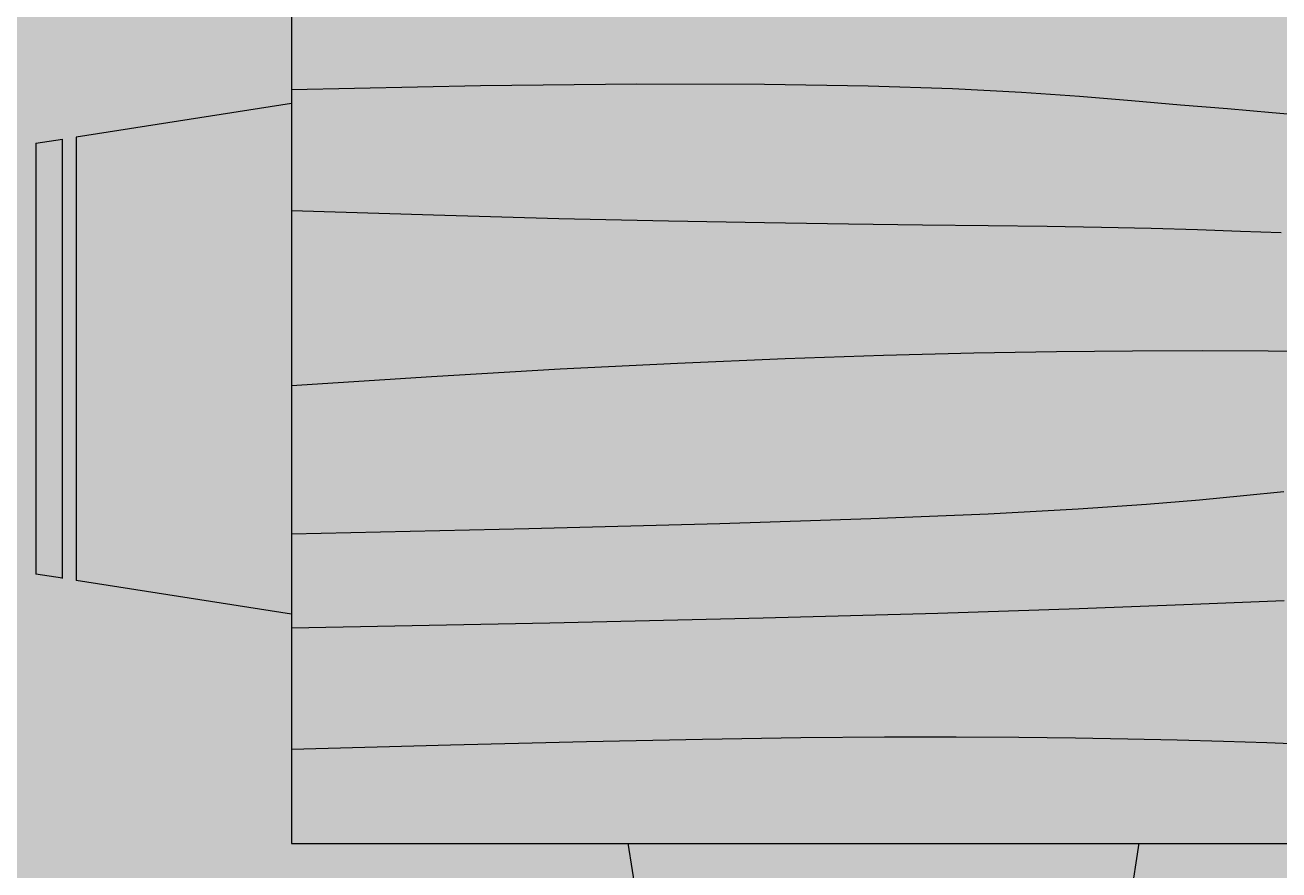
# Model space of a CAD drawing. Units: inches. Extents: x 3024 to 3952, y 1308 to 1863.
# Tile 8 of 29: x 3323 to 3357, y 1587 to 1610. Entities that reach past the tile are written whole.
import ezdxf

# ---------------------------------------------------------------- set-up
doc = ezdxf.new("R2010")
doc.units = ezdxf.units.IN
for name, color, linetype, lineweight in [('A-ANNO-DIMS', 2, 'Continuous', 18), ('A-FLOR-TILE-PATT', 7, 'Continuous', 13), ('A-FURN', 8, 'Continuous', 18), ('A-FURN-PATT', 9, 'Continuous', 13)]:
    doc.layers.add(name, color=color, linetype=linetype, lineweight=lineweight)
doc.layers.add('A-FLOR-PATT', color=254, linetype='Continuous', lineweight=13, true_color=0xfeeab9)
doc.styles.get("Standard").update_dxf_attribs({"font": 'arial.ttf'})
doc.dimstyles.get("Standard").update_dxf_attribs({"dimtxt": 0.18, "dimasz": 0.18, "dimexe": 0.18, "dimexo": 0.0625, "dimgap": 0.09, "dimtad": 0, "dimtih": 1, "dimtoh": 1, "dimdec": 4, "dimzin": 0, "dimdsep": 46, "dimtxsty": 'Standard', "dimcen": 0.09, "dimadec": 0, "dimazin": 0, "dimtfac": 1, "dimtdec": 4, "dimtofl": 0, "dimtmove": 0, "dimatfit": 3, "dimfxl": 1, "dimtolj": 1, "dimtzin": 0, "dimarcsym": 0})

# ---------------------------------------------------------------- blocks, each defined once
blk = doc.blocks.new('Dining Set - 36 x 72 in.')
for p, q in [((-36, 18), (-36, -18)), ((-44.0006, 8.23428), (-35.9976, 9.48474)), ((-45.5, 8), (-44.5004, 8.15617)), ((-45.5, 8), (-45.5, -8)), ((-44.5, -8.15843), (-44.5, 8.15338)), ((-44, 8.23041), (-44, -8.23915)), ((-44.4997, -8.15631), (-45.5, -8)), ((-35.9976, -9.48476), (-43.9993, -8.2345)), ((-36, -18), (36, -18)), ((-22.2343, -26.0006), (-23.4847, -17.99762)), ((-4.5152, -17.99762), (-5.7655, -25.99928))]:
    blk.add_line(p, q)
for points in [[(-36, 10), (-28.9766, 10.14274), (-23.1725, 10.20442), (-18.4241, 10.19775), (-14.5677, 10.13541), (-11.4399, 10.03011), (-8.877, 9.89453), (-6.7154, 9.74137), (-4.7917, 9.58333), (-2.9698, 9.43082), (-1.2246, 9.28515), (0.4415, 9.14534), (2.026, 9.01041)], [(-36, 5.5), (-30.7157, 5.3348), (-26.069, 5.20963), (-21.9946, 5.11767), (-18.4271, 5.05208), (-15.3009, 5.00602), (-12.5508, 4.97265), (-10.1112, 4.94515), (-7.9167, 4.91666), (-5.909, 4.88167), (-4.0586, 4.83984), (-2.3429, 4.79215), (-0.7396, 4.73958), (0.7739, 4.6831)], [(-36, -1), (-30.7915, -0.6591), (-26.0195, -0.38216), (-21.6519, -0.16284), (-17.6563, 0.00521), (-14.0005, 0.12833), (-10.6523, 0.21289), (-7.5796, 0.26522), (-4.75, 0.29166), (-2.134, 0.29793), (0.2878, 0.28711), (2.5317, 0.26163)], [(-36, -6.5), (-27.1843, -6.31267), (-20.084, -6.1263), (-14.469, -5.9419), (-10.1094, -5.76042), (-6.7752, -5.58285), (-4.2363, -5.41016), (-2.2629, -5.24333), (-0.625, -5.08334), (0.8708, -4.93099)], [(-36, -10), (-26.4022, -9.81299), (-18.4675, -9.62891), (-11.9839, -9.45069), (-6.7396, -9.28125), (-2.5226, -9.12354), (0.8789, -8.98047)], [(-36, -14.5), (-30.0881, -14.33513), (-25.0332, -14.21224), (-20.7312, -14.12647), (-17.0781, -14.07292), (-13.97, -14.04671), (-11.3027, -14.04297), (-8.9724, -14.05681), (-6.875, -14.08334), (-4.9224, -14.11833), (-3.0905, -14.16016), (-1.3709, -14.20785), (0.2448, -14.26042), (1.7647, -14.3169)]]:
    blk.add_lwpolyline(points)
blk = doc.blocks.new('*D21')
at = {"layer": 'A-ANNO-DIMS', "color": 0, "lineweight": -2, "transparency": 16777216}
for p, q in [((3323.055, 1621.114), (3312.873, 1621.114)), ((3313.053, 1620.934), (3313.053, 1601.018)), ((3313.053, 1580.742), (3313.053, 1600.657)), ((3323.055, 1580.562), (3312.873, 1580.562))]:
    blk.add_line(p, q, dxfattribs=at)
at = {"layer": 'A-ANNO-DIMS', "color": 0, "transparency": 16777216}
for points in [[(3313.023, 1620.934), (3313.083, 1620.934), (3313.053, 1621.114)], [(3313.023, 1580.742), (3313.083, 1580.742), (3313.053, 1580.562)]]:
    blk.add_solid(points, dxfattribs=at)
at = {"layer": 'Defpoints', "color": 0, "transparency": 16777216}
for p in [(3313.053, 1621.114), (3323.117, 1621.114), (3323.117, 1580.562)]:
    blk.add_point(p, dxfattribs=at)
at = {"layer": 'A-ANNO-DIMS', "color": 0, "transparency": 16777216, "insert": (3313.053, 1600.838), "char_height": 0.18, "attachment_point": 5}
blk.add_mtext('\\A1;41', dxfattribs=at)

msp = doc.modelspace()

# ---------------------------------------------------------------- hatches: boundary and pattern name
at = {"layer": 'A-FLOR-PATT', "transparency": 33554528}
h = msp.add_hatch(color=256, dxfattribs=at)
h.dxf.hatch_style = 1
h.paths.add_polyline_path([(3460.764, 1688.6064), (3412.764, 1688.6064), (3412.764, 1694.6064), (3460.764, 1694.6064), (3460.764, 1778.6064), (3406.764, 1778.6064), (3406.764, 1759.9514), (3318.2981, 1759.9514), (3318.2981, 1658.6064), (3322.5356, 1658.6064), (3322.5356, 1652.6064), (3292.764, 1652.6064), (3292.764, 1778.6064), (3106.764, 1778.6064), (3106.764, 1628.6064), (3172.764, 1628.6064), (3172.764, 1532.6064), (3166.764, 1532.6064), (3166.764, 1628.6064), (3106.764, 1628.6064), (3106.764, 1356.8452), (3202.812, 1356.8452), (3202.812, 1354.2534), (3202.812, 1353.8388), (3202.812, 1351.1212), (3202.812, 1347.8452), (3277.764, 1347.8452), (3277.764, 1353.8452), (3277.764, 1356.8452), (3277.764, 1442.6064), (3460.764, 1442.6064)])
h.paths.add_polyline_path([(3216.238, 1527.2064), (3216.238, 1491.2064), (3214.663, 1491.2064), (3214.663, 1491.2409, -0.3966224), (3180.243, 1526.6064), (3163.0285, 1526.6064), (3163.0285, 1531.1064), (3161.716, 1531.1064), (3161.716, 1561.1064), (3163.0285, 1561.1064), (3163.0285, 1531.1064), (3163.0285, 1526.6064), (3180.243, 1526.6064, 0.3966224), (3214.663, 1491.2409), (3214.663, 1527.2064)], flags=16)
h.paths.add_polyline_path([(3227.364, 1649.8972), (3191.364, 1649.8972), (3191.364, 1651.4722), (3227.364, 1651.4722)], flags=16)
h.paths.add_polyline_path([(3323.1172, 1606.7362), (3323.8545, 1606.8514), (3323.8545, 1594.8241), (3323.1172, 1594.9393)], flags=16)
h.paths.add_polyline_path([(3324.2232, 1606.909), (3330.1216, 1607.8307), (3330.1216, 1614.1093), (3339.3495, 1614.1093), (3340.2711, 1620.0078), (3352.4136, 1620.0078), (3353.3353, 1614.1093), (3359.9941, 1614.1093), (3360.9157, 1620.0078), (3373.0582, 1620.0078), (3373.9799, 1614.1093), (3383.2077, 1614.1093), (3383.2077, 1607.8307), (3389.1062, 1606.909), (3389.1062, 1594.7665), (3383.2077, 1593.8449), (3383.2077, 1587.5663), (3373.9799, 1587.5663), (3373.0583, 1581.6678), (3360.9157, 1581.6678), (3359.9941, 1587.5663), (3353.3353, 1587.5663), (3352.4136, 1581.6678), (3340.2711, 1581.6678), (3339.3495, 1587.5663), (3330.1216, 1587.5663), (3330.1216, 1593.8449), (3324.2232, 1594.7665)], flags=16)
h.paths.add_polyline_path([(3236.1584, 1693.1064), (3236.1584, 1723.1064), (3237.4709, 1723.1064), (3237.4709, 1693.1064)], flags=16)
h.paths.add_polyline_path([(3373.2158, 1600.6847), (3373.7965, 1600.7303), (3374.3268, 1600.7874), (3374.8132, 1600.8531), (3375.2621, 1600.9247), (3375.6801, 1600.9991), (3376.0736, 1601.0735), (3376.6855, 1601.19), (3377.366, 1601.3023), (3378.0667, 1601.3814), (3378.8026, 1601.4123), (3379.5865, 1601.3839), (3380.4537, 1601.2948), (3381.301, 1601.1717), (3382.0317, 1601.0433), (3382.4398, 1600.9607), (3382.6252, 1600.9201), (3382.919, 1600.8507), (3382.9044, 1600.8531), (3382.842, 1600.8678), (3382.7541, 1600.8896), (3382.6252, 1600.9201), (3382.4398, 1600.9607), (3382.1868, 1601.0119), (3381.8738, 1601.0711), (3381.5125, 1601.1346), (3381.1149, 1601.1988), (3380.6928, 1601.2601), (3380.2581, 1601.3149), (3379.8226, 1601.3597), (3379.3984, 1601.3908), (3378.9944, 1601.4054), (3378.6092, 1601.4042), (3378.2384, 1601.3886), (3377.8777, 1601.36), (3377.5227, 1601.32), (3377.1691, 1601.2698), (3376.8127, 1601.211), (3376.4491, 1601.145), (3376.0736, 1601.0735), (3375.4177, 1600.9494), (3374.5542, 1600.8119), (3373.5044, 1600.6988)], flags=0)
h.paths.add_polyline_path([(3380.0253, 1596.7351), (3380.499, 1596.6659), (3380.9706, 1596.6119), (3381.4375, 1596.5791), (3381.8971, 1596.5736), (3382.5886, 1596.6167), (3382.7848, 1596.6692), (3382.1465, 1596.5706), (3381.236, 1596.5815), (3380.3199, 1596.6865)], flags=0)
h.paths.add_polyline_path([(3369.6414, 1603.9617), (3370.1589, 1604.0021), (3370.6218, 1604.0539), (3371.0335, 1604.1173), (3371.3978, 1604.1921), (3371.7181, 1604.2785), (3371.9984, 1604.3761), (3372.2441, 1604.483), (3372.4611, 1604.5972), (3372.655, 1604.7163), (3372.8317, 1604.8384), (3372.9968, 1604.9611), (3373.3703, 1605.2455), (3373.8426, 1605.5328), (3374.4624, 1605.7539), (3375.1058, 1605.8302), (3375.7221, 1605.8261), (3376.4109, 1605.76), (3377.1534, 1605.6376), (3377.8945, 1605.473), (3378.1382, 1605.409), (3377.7394, 1605.5074), (3377.3509, 1605.5937), (3376.9704, 1605.6677), (3376.5999, 1605.7288), (3376.2417, 1605.7762), (3375.8979, 1605.8092), (3375.5707, 1605.8271), (3375.2621, 1605.8291), (3374.9745, 1605.8146), (3374.7092, 1605.7832), (3374.4647, 1605.7359), (3374.239, 1605.6742), (3374.0298, 1605.5996), (3373.835, 1605.5134), (3373.6525, 1605.4171), (3373.4801, 1605.3123), (3373.3156, 1605.2002), (3373.1562, 1605.0825), (3372.7603, 1604.781), (3372.236, 1604.4588), (3371.5738, 1604.2283), (3370.8493, 1604.0794), (3369.9262, 1603.976)], flags=0)
h.paths.add_polyline_path([(3366.7533, 1606.5832), (3367.1713, 1606.5519), (3367.5378, 1606.5374), (3367.8568, 1606.5394), (3368.1325, 1606.5573), (3368.3694, 1606.5903), (3368.5717, 1606.6377), (3368.7438, 1606.6988), (3368.89, 1606.7728), (3369.0146, 1606.8591), (3369.121, 1606.9568), (3369.2094, 1607.0646), (3369.2792, 1607.181), (3369.3295, 1607.3046), (3369.3596, 1607.4339), (3369.3688, 1607.5676), (3369.3565, 1607.7042), (3369.3218, 1607.8422), (3369.2649, 1607.9804), (3369.1893, 1608.1187), (3369.0993, 1608.2569), (3368.9992, 1608.3952), (3368.8934, 1608.5334), (3368.7861, 1608.6717), (3368.6817, 1608.8099), (3368.4212, 1609.1804), (3368.2685, 1609.7106), (3368.4883, 1610.1814), (3369.0537, 1610.4604), (3369.6717, 1610.5097), (3370.2812, 1610.3612), (3370.4805, 1610.2968), (3370.1882, 1610.3839), (3369.9284, 1610.4472), (3369.6905, 1610.4842), (3369.4662, 1610.4933), (3369.2555, 1610.4765), (3369.0608, 1610.4367), (3368.884, 1610.3767), (3368.7274, 1610.2994), (3368.5931, 1610.2077), (3368.4833, 1610.1045), (3368.4002, 1609.9927), (3368.3451, 1609.8747), (3368.3166, 1609.7517), (3368.3127, 1609.6244), (3368.331, 1609.4935), (3368.3696, 1609.3597), (3368.4261, 1609.2237), (3368.4985, 1609.0863), (3368.5845, 1608.9482), (3368.6817, 1608.8099), (3368.7861, 1608.6717), (3368.8934, 1608.5334), (3368.9992, 1608.3952), (3369.0993, 1608.2569), (3369.3398, 1607.8876), (3369.3941, 1607.2896), (3368.9774, 1606.7817), (3368.3928, 1606.5742), (3367.7162, 1606.5303), (3367.0044, 1606.5585)], flags=0)
h.paths.add_polyline_path([(3362.1859, 1610.2589), (3362.5478, 1610.2845), (3362.8348, 1610.3275), (3363.0585, 1610.3863), (3363.2303, 1610.4595), (3363.3619, 1610.5457), (3363.463, 1610.6432), (3363.5376, 1610.7502), (3363.5876, 1610.8643), (3363.6153, 1610.9834), (3363.6229, 1611.1055), (3363.6125, 1611.2283), (3363.5861, 1611.3496), (3363.5462, 1611.4673), (3363.4949, 1611.5797), (3363.4358, 1611.6871), (3363.3723, 1611.7902), (3363.3081, 1611.8897), (3363.2468, 1611.9863), (3363.192, 1612.0808), (3363.0258, 1612.4261), (3363.3371, 1612.8672), (3363.9008, 1612.9782), (3364.4822, 1612.9641), (3365.1098, 1612.9074), (3365.328, 1612.8805), (3364.9615, 1612.9208), (3364.6426, 1612.9496), (3364.3668, 1612.9669), (3364.1299, 1612.9726), (3363.9276, 1612.9669), (3363.7555, 1612.9496), (3363.6093, 1612.9208), (3363.4848, 1612.8805), (3363.3782, 1612.8289), (3363.2889, 1612.7672), (3363.2169, 1612.6969), (3363.1622, 1612.6193), (3363.1247, 1612.5361), (3363.1046, 1612.4484), (3363.1017, 1612.358), (3363.1161, 1612.266), (3363.1472, 1612.1738), (3363.192, 1612.0808), (3363.2468, 1611.9863), (3363.3081, 1611.8897), (3363.3723, 1611.7902), (3363.4358, 1611.6871), (3363.6363, 1611.323), (3363.5979, 1610.7003), (3363.0863, 1610.3651), (3362.3983, 1610.2622)], flags=0)
h.paths.add_polyline_path([(3352.356, 1581.2991), (3352.2408, 1580.5618), (3340.4439, 1580.5618), (3340.3287, 1581.2991)], flags=16)
h.paths.add_polyline_path([(3340.4439, 1621.1137), (3352.2408, 1621.1137), (3352.356, 1620.3764), (3340.3287, 1620.3764)], flags=16)
h.paths.add_polyline_path([(3278.4282, 1504.7424), (3290.3831, 1504.7424), (3290.3831, 1502.7499), (3291.0473, 1502.7499), (3291.0473, 1494.7799), (3290.3831, 1494.7799), (3290.3831, 1494.1158), (3291.0473, 1494.1158), (3291.0473, 1486.1458), (3290.3831, 1486.1458), (3290.3831, 1484.1533), (3291.0473, 1484.1533), (3291.0473, 1483.4892, -0.0909091), (3291.0473, 1468.8776), (3291.0473, 1468.2135), (3290.3831, 1468.2135), (3290.3831, 1464.8926), (3278.4282, 1464.8926), (3278.4282, 1472.8626), (3277.764, 1473.5268), (3277.764, 1478.84), (3278.4282, 1479.5042)], flags=16)
h.paths.add_polyline_path([(3278.7603, 1504.4103), (3290.051, 1504.4103), (3290.051, 1465.2247), (3278.7603, 1465.2247)], flags=0)
h.paths.add_polyline_path([(3123.904, 1600.7821), (3117.9039, 1602.7821), (3117.9039, 1599.7821), (3119.4039, 1599.7821), (3119.4039, 1596.7821), (3118.4039, 1596.7821), (3118.4039, 1598.7821), (3117.9039, 1598.7821), (3117.9039, 1596.2821), (3109.9039, 1596.2821), (3109.9039, 1617.2821), (3117.9039, 1617.2821), (3117.9039, 1610.7821), (3123.9038, 1612.7821, -0.7025712), (3137.9039, 1606.7822, -0.7025621)], flags=16)
h.paths.add_polyline_path([(3123.9039, 1602.7822), (3123.9039, 1610.7822, -0.7345333), (3136.9039, 1606.7822, -0.7345297)], flags=0)
h.paths.add_polyline_path([(3177.972, 1689.6473), (3109.2405, 1689.6473), (3109.2405, 1741.1959), (3177.972, 1741.1959)], flags=16)
h.paths.add_polyline_path([(3373.0006, 1581.2991), (3372.8854, 1580.5618), (3361.0885, 1580.5618), (3360.9733, 1581.2991)], flags=16)
h.paths.add_polyline_path([(3361.0885, 1621.1137), (3372.8854, 1621.1137), (3373.0006, 1620.3764), (3360.9733, 1620.3764)], flags=16)
h.paths.add_polyline_path([(3116.9039, 1598.2821, -0.4142136), (3116.1539, 1597.2821), (3111.9039, 1597.2821, -0.4142136), (3110.9039, 1598.0321), (3110.9039, 1615.2821, -0.4142136), (3111.6539, 1616.2821), (3115.9039, 1616.2821, -0.4142136), (3116.9039, 1615.5321)], flags=0)
h.paths.add_polyline_path([(3121.6122, 1728.1369), (3121.6122, 1696.5205), (3110.2715, 1696.5205), (3110.2715, 1714.3906), (3121.6122, 1714.3906), (3121.6122, 1716.4526), (3110.2715, 1716.4526), (3110.2715, 1734.3228), (3123.3304, 1734.3228), (3123.3304, 1729.8552), (3134.6711, 1741.1959), (3134.6711, 1728.1369)], flags=0)
h.paths.add_polyline_path([(3389.4748, 1606.8514), (3390.2122, 1606.7362), (3390.2122, 1594.9393), (3389.4748, 1594.8241)], flags=16)
h.paths.add_polyline_path([(3257.6842, 1762.8281), (3259.6842, 1768.8281), (3256.6842, 1768.8281), (3256.6842, 1767.3281), (3253.6842, 1767.3281), (3253.6842, 1768.3281), (3255.6842, 1768.3281), (3255.6842, 1768.8281), (3253.1842, 1768.8281), (3253.1842, 1776.8281), (3274.1842, 1776.8281), (3274.1842, 1768.8281), (3267.6842, 1768.8281), (3269.6842, 1762.8282, -0.7025712), (3263.6843, 1748.8282, -0.7025621)], flags=16)
h.paths.add_polyline_path([(3259.6842, 1762.8281), (3267.6843, 1762.8281, -0.7345333), (3263.6842, 1749.8282, -0.7345297)], flags=0)
h.paths.add_polyline_path([(3411.264, 1715.6064), (3411.264, 1716.9189), (3441.264, 1716.9189), (3441.264, 1715.6064)], flags=16)
h.paths.add_polyline_path([(3178.3806, 1449.1876), (3178.3806, 1397.639), (3109.6491, 1397.639), (3109.6491, 1449.1876)], flags=16)
h.paths.add_polyline_path([(3397.1501, 1541.7146), (3419.6183, 1541.7146), (3419.6183, 1496.7783), (3397.1501, 1496.7783)], flags=16)
h.paths.add_polyline_path([(3254.1842, 1770.5781), (3254.1842, 1774.8281, -0.4142136), (3254.9342, 1775.8281), (3272.1842, 1775.8281, -0.4142136), (3273.1842, 1775.0781), (3273.1842, 1770.8281, -0.4142136), (3272.4342, 1769.8281), (3255.1842, 1769.8281, -0.4142136)], flags=0)
h.paths.add_polyline_path([(3403.672, 1500.7601), (3403.6016, 1500.3997), (3403.5328, 1500.0441), (3403.4662, 1499.6867), (3403.4027, 1499.3226), (3403.3464, 1498.9532), (3403.3025, 1498.5811), (3403.2759, 1498.2091), (3403.2714, 1497.8401), (3403.3064, 1497.2813), (3403.3491, 1497.1219), (3403.2689, 1497.6395), (3403.2778, 1498.3719), (3403.3635, 1499.0984), (3403.4889, 1499.8168), (3403.6016, 1500.3997), (3403.672, 1500.7601), (3403.744, 1501.1315), (3403.817, 1501.5205), (3403.891, 1501.9336), (3403.9656, 1502.3769), (3404.0404, 1502.8572), (3404.115, 1503.3786), (3404.2264, 1504.2311), (3404.2571, 1504.5223), (3404.1552, 1503.6598), (3404.0063, 1502.6193), (3403.8604, 1501.7518), (3403.744, 1501.1315)], flags=0)
h.paths.add_polyline_path([(3406.5868, 1505.0416), (3406.6121, 1504.5236), (3406.6492, 1504.0526), (3406.6956, 1503.624), (3406.7491, 1503.2333), (3406.8072, 1502.8759), (3406.8676, 1502.5473), (3406.9281, 1502.243), (3407.0268, 1501.7597), (3407.1416, 1501.1368), (3407.2087, 1500.3904), (3407.1804, 1499.6703), (3407.1078, 1498.9956), (3407.0074, 1498.3199), (3406.8809, 1497.6059), (3406.7403, 1496.9627), (3406.7418, 1496.9824), (3406.7491, 1497.0249), (3406.8229, 1497.3409), (3406.8364, 1497.4025), (3406.878, 1497.6078), (3406.9261, 1497.8614), (3406.9777, 1498.1526), (3407.0298, 1498.4712), (3407.0797, 1498.8068), (3407.1243, 1499.149), (3407.1607, 1499.4874), (3407.1859, 1499.8115), (3407.1978, 1500.1137), (3407.1969, 1500.3962), (3407.1841, 1500.6642), (3407.1609, 1500.9225), (3407.1284, 1501.1761), (3407.0876, 1501.43), (3407.0398, 1501.6891), (3406.9862, 1501.9585), (3406.8832, 1502.4628), (3406.7712, 1503.0713), (3406.6657, 1503.8424), (3406.5924, 1504.7735)], flags=0)
h.paths.add_polyline_path([(3409.2517, 1507.8962), (3409.2752, 1507.4282), (3409.3079, 1507.0076), (3409.3501, 1506.6314), (3409.4015, 1506.2969), (3409.4624, 1506.0009), (3409.5326, 1505.7406), (3409.6119, 1505.5128), (3409.6988, 1505.3131), (3409.7915, 1505.1368), (3409.8883, 1504.9792), (3409.9875, 1504.8356), (3410.0872, 1504.7015), (3410.1859, 1504.572), (3410.4508, 1504.2132), (3410.7205, 1503.6035), (3410.8059, 1502.8824), (3410.7619, 1502.0875), (3410.6122, 1501.2299), (3410.4402, 1500.6169), (3410.2538, 1500.0031), (3410.0536, 1499.3219), (3409.9909, 1499.0812), (3410.1761, 1499.7472), (3410.3596, 1500.3513), (3410.4512, 1500.6561), (3410.5312, 1500.9412), (3410.6013, 1501.226), (3410.6614, 1501.512), (3410.7111, 1501.7964), (3410.7496, 1502.0763), (3410.7764, 1502.3489), (3410.7909, 1502.6114), (3410.7926, 1502.8608), (3410.7808, 1503.0944), (3410.7553, 1503.31), (3410.7169, 1503.5087), (3410.6667, 1503.6921), (3410.6061, 1503.8621), (3410.5361, 1504.0203), (3410.4578, 1504.1686), (3410.3726, 1504.3088), (3410.2815, 1504.4424), (3410.1859, 1504.572), (3410.0872, 1504.7015), (3409.859, 1505.0083), (3409.5943, 1505.5117), (3409.4266, 1506.1336), (3409.324, 1506.8011), (3409.2586, 1507.6407)], flags=0)
h.paths.add_polyline_path([(3411.4914, 1510.5878), (3411.4432, 1510.1586), (3411.4054, 1509.775), (3411.38, 1509.4354), (3411.3681, 1509.1376), (3411.3698, 1508.8784), (3411.3843, 1508.6542), (3411.4112, 1508.4618), (3411.4497, 1508.2974), (3411.4994, 1508.1575), (3411.5595, 1508.0388), (3411.6296, 1507.9375), (3411.7097, 1507.851), (3411.802, 1507.7792), (3411.9096, 1507.7225), (3412.0353, 1507.6817), (3412.1821, 1507.6572), (3412.3528, 1507.6496), (3412.5505, 1507.6597), (3412.778, 1507.6879), (3413.0364, 1507.7341), (3413.3194, 1507.7955), (3413.6188, 1507.8687), (3413.9264, 1507.95), (3414.234, 1508.036), (3414.5333, 1508.1232), (3414.8163, 1508.208), (3415.0747, 1508.287), (3415.3023, 1508.3569), (3415.5007, 1508.4158), (3415.6733, 1508.4617), (3416.1158, 1508.5538), (3416.512, 1508.2591), (3416.716, 1507.6581), (3416.61, 1507.0003), (3416.3052, 1506.3411), (3415.8928, 1505.618), (3415.7339, 1505.3633), (3415.9914, 1505.791), (3416.201, 1506.1583), (3416.3666, 1506.4739), (3416.4925, 1506.7462), (3416.5828, 1506.9838), (3416.6413, 1507.1949), (3416.6725, 1507.3883), (3416.6799, 1507.5705), (3416.6662, 1507.7417), (3416.6339, 1507.9), (3416.5851, 1508.0436), (3416.5223, 1508.1709), (3416.4478, 1508.28), (3416.3639, 1508.3692), (3416.273, 1508.4368), (3416.1765, 1508.4815), (3416.0718, 1508.5047), (3415.9553, 1508.5079), (3415.8237, 1508.493), (3415.6733, 1508.4617), (3415.5007, 1508.4158), (3415.3327, 1508.3659), (3414.6495, 1508.157), (3414.0606, 1507.9855), (3413.4456, 1507.8229), (3412.8838, 1507.701), (3412.5505, 1507.6597), (3412.0748, 1507.6354), (3411.595, 1507.8883), (3411.398, 1508.4429), (3411.3624, 1508.9927), (3411.3854, 1509.5711), (3411.4578, 1510.3071)], flags=0)
h.paths.add_polyline_path([(3135.0797, 1449.1876), (3135.0797, 1436.1286), (3122.0208, 1436.1286), (3122.0208, 1404.5122), (3110.6801, 1404.5122), (3110.6801, 1422.3823), (3122.0208, 1422.3823), (3122.0208, 1424.4443), (3110.6801, 1424.4443), (3110.6801, 1442.3145), (3123.739, 1442.3145), (3123.739, 1437.8469)], flags=0)
h.paths.add_polyline_path([(3416.4944, 1514.2949), (3416.4837, 1513.8511), (3416.4893, 1513.4867), (3416.5102, 1513.1926), (3416.5451, 1512.9593), (3416.5929, 1512.7775), (3416.6524, 1512.6379), (3416.7224, 1512.531), (3416.8017, 1512.4488), (3416.8886, 1512.3882), (3416.9813, 1512.3476), (3417.0781, 1512.3251), (3417.1773, 1512.3189), (3417.277, 1512.3274), (3417.3757, 1512.3488), (3417.4713, 1512.3813), (3417.5627, 1512.4229), (3417.65, 1512.471), (3417.7338, 1512.5225), (3417.8146, 1512.5747), (3417.8931, 1512.6245), (3417.9699, 1512.6691), (3418.2968, 1512.8265), (3418.6505, 1512.4645), (3418.7037, 1511.9342), (3418.6693, 1511.3839), (3418.6076, 1510.8228), (3418.5777, 1510.5927), (3418.6197, 1510.9333), (3418.6525, 1511.2311), (3418.6759, 1511.4903), (3418.6899, 1511.7144), (3418.6946, 1511.9069), (3418.6899, 1512.0713), (3418.6759, 1512.2112), (3418.6525, 1512.33), (3418.6197, 1512.4311), (3418.5778, 1512.5177), (3418.5276, 1512.5903), (3418.4705, 1512.6488), (3418.4075, 1512.6933), (3418.3399, 1512.7237), (3418.2686, 1512.7401), (3418.1951, 1512.7424), (3418.1204, 1512.7307), (3418.0455, 1512.7055), (3417.9792, 1512.6736), (3417.65, 1512.471), (3417.5627, 1512.4229), (3417.4713, 1512.3813), (3417.3757, 1512.3488), (3417.277, 1512.3274), (3416.878, 1512.2936), (3416.5757, 1512.7549), (3416.492, 1513.3145), (3416.4808, 1514.0384)], flags=0)
h.paths.add_polyline_path([(3392.8223, 1481.9454), (3396.7707, 1481.9454), (3396.7707, 1480.9201), (3428.3585, 1480.9201), (3428.3585, 1481.9454), (3432.3069, 1481.9454), (3432.3069, 1464.8354, -0.266667), (3392.8223, 1464.8354)], flags=16)
h.paths.add_polyline_path([(3431.203, 1547.5428), (3450.8613, 1547.5428, -0.1904762), (3450.8614, 1484.031), (3431.203, 1484.031), (3431.203, 1488.5675), (3432.3809, 1488.5675), (3432.3809, 1543.0062), (3431.203, 1543.0062)], flags=16)
h.paths.add_polyline_path([(3451.9233, 1524.86, -0.0496282), (3451.9233, 1506.7138), (3446.7921, 1506.7138), (3446.7921, 1524.86)], flags=0)
h.paths.add_polyline_path([(3460.764, 1436.6064), (3277.764, 1436.6064), (3277.764, 1356.8452), (3277.764, 1353.8452), (3460.764, 1353.8452)], flags=17)
h.paths.add_polyline_path([(3121.3033, 1577.378), (3153.693, 1577.378), (3153.693, 1586.6752), (3121.3033, 1586.6752)], flags=24)
h.paths.add_polyline_path([(3164.1457, 1464.1276), (3210.4801, 1464.1276), (3210.4801, 1473.4247), (3164.1457, 1473.4247)], flags=24)
h.paths.add_polyline_path([(3343.1909, 1505.8863), (3373.7236, 1505.8863), (3373.7236, 1515.1773), (3343.1909, 1515.1773)], flags=24)
h.paths.add_polyline_path([(3337.6353, 1564.2926), (3370.0189, 1564.2926), (3370.0189, 1573.5836), (3337.6353, 1573.5836)], flags=24)
h.paths.add_polyline_path([(3419.204, 1753.8578), (3453.3997, 1753.8578), (3453.3997, 1762.9956), (3419.204, 1762.9956)], flags=24)
h.paths.add_polyline_path([(3341.2523, 1701.0246), (3381.0761, 1701.0246), (3381.0761, 1710.3156), (3341.2523, 1710.3156)], flags=24)
h.paths.add_polyline_path([(3245.8895, 1726.2997), (3278.2793, 1726.2997), (3278.2793, 1735.5968), (3245.8895, 1735.5968)], flags=24)
h.paths.add_polyline_path([(3128.8045, 1668.6736), (3175.1389, 1668.6736), (3175.1389, 1677.9707), (3128.8045, 1677.9707)], flags=24)
h.paths.add_polyline_path([(3345.9997, 1396.0062), (3389.09, 1396.0062), (3389.09, 1405.3033), (3345.9997, 1405.3033)], flags=24)
at = {"layer": 'A-FLOR-TILE-PATT', "transparency": 33554569}
h = msp.add_hatch(dxfattribs=at)
h.set_pattern_fill('ANGLE', color=256, scale=2)
h.set_pattern_definition([(0, (0, 0), (0, 13.97), [10.16, -3.81]), (90, (0, 0), (-13.97, 9e-16), [10.16, -3.81])])
h.paths.add_polyline_path([(3292.764, 1778.6064), (3232.764, 1778.6064), (3232.764, 1694.6064), (3236.1584, 1694.6064), (3236.1584, 1723.1064), (3237.4709, 1723.1064), (3237.4709, 1723.0777, -0.3870039), (3266.1209, 1694.6064), (3292.764, 1694.6064)])
h.paths.add_polyline_path([(3263.6843, 1748.8282, -0.7025621), (3257.6842, 1762.8281), (3259.6842, 1768.8281), (3256.6842, 1768.8281), (3256.6842, 1767.3281), (3253.6842, 1767.3281), (3253.6842, 1768.3281), (3255.6842, 1768.3281), (3255.6842, 1768.8281), (3253.1842, 1768.8281), (3253.1842, 1776.8281), (3274.1842, 1776.8281), (3274.1842, 1768.8281), (3267.6842, 1768.8281), (3269.6842, 1762.8282, -0.7025712)], flags=16)
h.paths.add_polyline_path([(3263.6842, 1749.8282, -0.7345297), (3259.6842, 1762.8281), (3267.6843, 1762.8281, -0.7345333)], flags=0)
h.paths.add_polyline_path([(3255.1842, 1769.8281, -0.4142136), (3254.1842, 1770.5781), (3254.1842, 1774.8281, -0.4142136), (3254.9342, 1775.8281), (3272.1842, 1775.8281, -0.4142136), (3273.1842, 1775.0781), (3273.1842, 1770.8281, -0.4142136), (3272.4342, 1769.8281)], flags=0)
h.paths.add_polyline_path([(3460.764, 1436.6064), (3277.764, 1436.6064), (3277.764, 1356.8452), (3277.764, 1353.8452), (3460.764, 1353.8452)])
h.paths.add_polyline_path([(3166.764, 1628.6064), (3106.764, 1628.6064), (3106.764, 1532.6064), (3133.066, 1532.6064, -0.3870039), (3161.716, 1561.0777), (3161.716, 1561.1064), (3163.0285, 1561.1064), (3163.0285, 1532.6064), (3166.764, 1532.6064)])
h.paths.add_polyline_path([(3123.904, 1600.7821), (3117.9039, 1602.7821), (3117.9039, 1599.7821), (3119.4039, 1599.7821), (3119.4039, 1596.7821), (3118.4039, 1596.7821), (3118.4039, 1598.7821), (3117.9039, 1598.7821), (3117.9039, 1596.2821), (3109.9039, 1596.2821), (3109.9039, 1617.2821), (3117.9039, 1617.2821), (3117.9039, 1610.7821), (3123.9038, 1612.7821, -0.7025712), (3137.9039, 1606.7822, -0.7025621)], flags=16)
h.paths.add_polyline_path([(3123.9039, 1602.7822), (3123.9039, 1610.7822, -0.7345333), (3136.9039, 1606.7822, -0.7345297)], flags=0)
h.paths.add_polyline_path([(3116.1539, 1597.2821), (3111.9039, 1597.2821, -0.4142136), (3110.9039, 1598.0321), (3110.9039, 1615.2821, -0.4142136), (3111.6539, 1616.2821), (3115.9039, 1616.2821, -0.4142136), (3116.9039, 1615.5321), (3116.9039, 1598.2821, -0.4142136)], flags=0)
h.paths.add_polyline_path([(3245.8895, 1726.2997), (3278.2793, 1726.2997), (3278.2793, 1735.5968), (3245.8895, 1735.5968)], flags=24)
h.paths.add_polyline_path([(3345.9997, 1396.0062), (3389.09, 1396.0062), (3389.09, 1405.3033), (3345.9997, 1405.3033)], flags=24)
h.paths.add_polyline_path([(3121.3033, 1577.378), (3153.693, 1577.378), (3153.693, 1586.6752), (3121.3033, 1586.6752)], flags=24)
at = {"layer": 'A-FURN-PATT', "transparency": 33554511}
h = msp.add_hatch(color=256, dxfattribs=at)
h.dxf.hatch_style = 1
h.paths.add_polyline_path([(3373.0582, 1620.0078), (3360.9157, 1620.0078), (3359.9941, 1614.1093), (3373.9799, 1614.1093)])
h.paths.add_polyline_path([(3372.8854, 1621.1137), (3361.0885, 1621.1137), (3360.9733, 1620.3764), (3373.0006, 1620.3764)])
h.paths.add_polyline_path([(3389.1062, 1606.909), (3383.2077, 1607.8307), (3383.2077, 1593.8449), (3389.1062, 1594.7665)])
h.paths.add_polyline_path([(3390.2122, 1606.7362), (3389.4748, 1606.8514), (3389.4748, 1594.8241), (3390.2122, 1594.9393)])
h.paths.add_polyline_path([(3373.9799, 1587.5663), (3359.9941, 1587.5663), (3360.9157, 1581.6678), (3373.0583, 1581.6678)])
h.paths.add_polyline_path([(3373.0006, 1581.2991), (3360.9733, 1581.2991), (3361.0885, 1580.5618), (3372.8854, 1580.5618)])
h.paths.add_polyline_path([(3353.3353, 1587.5663), (3339.3495, 1587.5663), (3340.2711, 1581.6678), (3352.4136, 1581.6678)])
h.paths.add_polyline_path([(3352.356, 1581.2991), (3340.3287, 1581.2991), (3340.4439, 1580.5618), (3352.2408, 1580.5618)])
h.paths.add_polyline_path([(3330.1216, 1607.8307), (3324.2232, 1606.909), (3324.2232, 1594.7665), (3330.1216, 1593.8449)])
h.paths.add_polyline_path([(3323.8545, 1606.8514), (3323.1172, 1606.7362), (3323.1172, 1594.9393), (3323.8545, 1594.8241)])
h.paths.add_polyline_path([(3352.4136, 1620.0078), (3340.2711, 1620.0078), (3339.3495, 1614.1093), (3353.3353, 1614.1093)])
h.paths.add_polyline_path([(3352.2408, 1621.1137), (3340.4439, 1621.1137), (3340.3287, 1620.3764), (3352.356, 1620.3764)])
at = {"layer": 'A-FURN-PATT', "transparency": 33554600}
h = msp.add_hatch(color=256, dxfattribs=at)
h.dxf.hatch_style = 1
h.paths.add_polyline_path([(3363.5462, 1611.4673), (3363.4949, 1611.5797), (3363.4358, 1611.6871), (3363.3723, 1611.7902), (3363.2557, 1611.9708), (3363.16, 1612.1359), (3363.1003, 1612.3129), (3363.1061, 1612.4946), (3363.1815, 1612.6623), (3363.3264, 1612.8038), (3363.5397, 1612.9071), (3363.7555, 1612.9496), (3363.9276, 1612.9669), (3364.1299, 1612.9726), (3364.3668, 1612.9669), (3364.6426, 1612.9496), (3364.9615, 1612.9208), (3365.328, 1612.8805), (3365.7471, 1612.8287), (3366.2271, 1612.7662), (3366.7769, 1612.6936), (3367.4055, 1612.6117), (3368.1221, 1612.5211), (3368.9354, 1612.4225), (3369.8546, 1612.3168), (3370.8886, 1612.2046), (3372.0442, 1612.0866), (3373.3189, 1611.9636), (3374.7081, 1611.8363), (3376.2072, 1611.7054), (3377.8113, 1611.5716), (3379.516, 1611.4356), (3381.3163, 1611.2982), (3383.2077, 1611.1601), (3383.2077, 1614.1093), (3330.1216, 1614.1093), (3330.1216, 1611.8974), (3333.6775, 1611.8808), (3336.899, 1611.834), (3339.8144, 1611.7613), (3342.4523, 1611.667), (3344.8411, 1611.5554), (3347.0091, 1611.4308), (3348.985, 1611.2976), (3350.797, 1611.1601), (3352.4691, 1611.0223), (3354.0078, 1610.8874), (3355.4146, 1610.7583), (3356.6916, 1610.6378), (3357.8403, 1610.5289), (3358.8627, 1610.4343), (3359.7605, 1610.357), (3360.5355, 1610.2999), (3361.1912, 1610.2651), (3361.7375, 1610.2519), (3362.1859, 1610.2589), (3362.5478, 1610.2845), (3362.8348, 1610.3275), (3363.0585, 1610.3863), (3363.2303, 1610.4595), (3363.3619, 1610.5457), (3363.463, 1610.6432), (3363.5376, 1610.7502), (3363.5876, 1610.8643), (3363.6153, 1610.9834), (3363.6229, 1611.1055), (3363.6125, 1611.2283), (3363.5861, 1611.3496)])
h.paths.add_polyline_path([(3368.8934, 1608.5334), (3368.7093, 1608.7706), (3368.5315, 1609.0235), (3368.3879, 1609.2961), (3368.3108, 1609.5637), (3368.3187, 1609.8182), (3368.4002, 1609.9927), (3368.4833, 1610.1045), (3368.5931, 1610.2077), (3368.7274, 1610.2994), (3368.884, 1610.3767), (3369.0608, 1610.4367), (3369.2555, 1610.4765), (3369.4662, 1610.4933), (3369.6905, 1610.4842), (3369.9284, 1610.4472), (3370.1882, 1610.3839), (3370.4805, 1610.2968), (3370.8156, 1610.1885), (3371.204, 1610.0615), (3371.6561, 1609.9183), (3372.1824, 1609.7614), (3372.7933, 1609.5933), (3373.5016, 1609.4153), (3374.3298, 1609.2232), (3375.3028, 1609.0117), (3376.4453, 1608.7754), (3377.7822, 1608.5088), (3379.3383, 1608.2065), (3381.1386, 1607.8633), (3383.2077, 1607.4735), (3383.2077, 1611.1601), (3381.3163, 1611.2982), (3379.516, 1611.4356), (3377.8113, 1611.5716), (3376.2072, 1611.7054), (3374.7081, 1611.8363), (3373.3189, 1611.9636), (3372.0442, 1612.0866), (3370.8886, 1612.2046), (3369.8546, 1612.3168), (3368.9354, 1612.4225), (3368.1221, 1612.5211), (3367.4055, 1612.6117), (3366.7769, 1612.6936), (3366.2271, 1612.7662), (3365.7471, 1612.8287), (3365.328, 1612.8805), (3364.9615, 1612.9208), (3364.6426, 1612.9496), (3364.3668, 1612.9669), (3364.1299, 1612.9726), (3363.9276, 1612.9669), (3363.7555, 1612.9496), (3363.6093, 1612.9208), (3363.4848, 1612.8805), (3363.3782, 1612.8289), (3363.2889, 1612.7672), (3363.2169, 1612.6969), (3363.1622, 1612.6193), (3363.1247, 1612.5361), (3363.1046, 1612.4484), (3363.1017, 1612.358), (3363.1161, 1612.266), (3363.1472, 1612.1738), (3363.192, 1612.0808), (3363.2468, 1611.9863), (3363.3081, 1611.8897), (3363.4181, 1611.7194), (3363.529, 1611.5178), (3363.6075, 1611.2866), (3363.6284, 1611.0397), (3363.5728, 1610.8008), (3363.4229, 1610.5856), (3363.2303, 1610.4595), (3363.0585, 1610.3863), (3362.8348, 1610.3275), (3362.5478, 1610.2845), (3362.1859, 1610.2589), (3361.7375, 1610.2519), (3361.1912, 1610.2651), (3360.5355, 1610.2999), (3359.7605, 1610.357), (3358.8627, 1610.4343), (3357.8403, 1610.5289), (3356.6916, 1610.6378), (3355.4146, 1610.7583), (3354.0078, 1610.8874), (3352.4691, 1611.0223), (3350.797, 1611.1601), (3348.985, 1611.2976), (3347.0091, 1611.4308), (3344.8411, 1611.5554), (3342.4523, 1611.667), (3339.8144, 1611.7613), (3336.899, 1611.834), (3333.6775, 1611.8808), (3330.1216, 1611.8974), (3330.1216, 1608.2109), (3335.3, 1608.3161), (3339.5794, 1608.3616), (3343.0805, 1608.3567), (3345.9238, 1608.3107), (3348.23, 1608.2331), (3350.1196, 1608.1331), (3351.7134, 1608.0202), (3353.1317, 1607.9036), (3354.475, 1607.7912), (3355.7618, 1607.6838), (3356.9902, 1607.5807), (3358.1585, 1607.4812), (3359.2649, 1607.3846), (3360.3076, 1607.2902), (3361.2846, 1607.1972), (3362.1945, 1607.1049), (3363.0358, 1607.0131), (3363.8102, 1606.9234), (3364.5198, 1606.8381), (3365.1667, 1606.7593), (3365.7532, 1606.6891), (3366.2814, 1606.6297), (3366.7533, 1606.5832), (3367.1713, 1606.5519), (3367.5378, 1606.5374), (3367.8568, 1606.5394), (3368.1325, 1606.5573), (3368.3694, 1606.5903), (3368.5717, 1606.6377), (3368.7438, 1606.6988), (3368.89, 1606.7728), (3369.0146, 1606.8591), (3369.121, 1606.9568), (3369.2094, 1607.0646), (3369.2792, 1607.181), (3369.3295, 1607.3046), (3369.3596, 1607.4339), (3369.3688, 1607.5676), (3369.3565, 1607.7042), (3369.3218, 1607.8422), (3369.2649, 1607.9804), (3369.1893, 1608.1187), (3369.0993, 1608.2569), (3368.9992, 1608.3952)])
h.paths.add_polyline_path([(3374.239, 1605.6742), (3374.4647, 1605.7359), (3374.7092, 1605.7832), (3374.9745, 1605.8146), (3375.2621, 1605.8291), (3375.5707, 1605.8271), (3375.8979, 1605.8092), (3376.2417, 1605.7762), (3376.5999, 1605.7288), (3376.9704, 1605.6677), (3377.3509, 1605.5937), (3377.7394, 1605.5074), (3378.1382, 1605.409), (3378.5679, 1605.2962), (3379.0538, 1605.1661), (3379.621, 1605.0159), (3380.2949, 1604.8426), (3381.1005, 1604.6434), (3382.0631, 1604.4154), (3383.2077, 1604.1557), (3383.2077, 1607.4735), (3381.1386, 1607.8633), (3379.3383, 1608.2065), (3377.7822, 1608.5088), (3376.4453, 1608.7754), (3375.3028, 1609.0117), (3374.3298, 1609.2232), (3373.5016, 1609.4153), (3372.7933, 1609.5933), (3372.1824, 1609.7614), (3371.6561, 1609.9183), (3371.204, 1610.0615), (3370.8156, 1610.1885), (3370.4805, 1610.2968), (3370.1882, 1610.3839), (3369.9284, 1610.4472), (3369.6905, 1610.4842), (3369.4662, 1610.4933), (3369.2555, 1610.4765), (3369.0608, 1610.4367), (3368.884, 1610.3767), (3368.7274, 1610.2994), (3368.5931, 1610.2077), (3368.4833, 1610.1045), (3368.4002, 1609.9927), (3368.3451, 1609.8747), (3368.3166, 1609.7517), (3368.3127, 1609.6244), (3368.331, 1609.4935), (3368.3696, 1609.3597), (3368.4261, 1609.2237), (3368.4985, 1609.0863), (3368.5845, 1608.9482), (3368.6817, 1608.8099), (3368.7861, 1608.6717), (3368.9798, 1608.422), (3369.1584, 1608.1753), (3369.306, 1607.9053), (3369.3736, 1607.6361), (3369.355, 1607.3674), (3369.2539, 1607.1187), (3369.121, 1606.9568), (3369.0146, 1606.8591), (3368.89, 1606.7728), (3368.7438, 1606.6988), (3368.5717, 1606.6377), (3368.3694, 1606.5903), (3368.1325, 1606.5573), (3367.8568, 1606.5394), (3367.5378, 1606.5374), (3367.1713, 1606.5519), (3366.7533, 1606.5832), (3366.2814, 1606.6297), (3365.7532, 1606.6891), (3365.1667, 1606.7593), (3364.5198, 1606.8381), (3363.8102, 1606.9234), (3363.0358, 1607.0131), (3362.1945, 1607.1049), (3361.2846, 1607.1972), (3360.3076, 1607.2902), (3359.2649, 1607.3846), (3358.1585, 1607.4812), (3356.9902, 1607.5807), (3355.7618, 1607.6838), (3354.475, 1607.7912), (3353.1317, 1607.9036), (3351.7134, 1608.0202), (3350.1196, 1608.1331), (3348.23, 1608.2331), (3345.9238, 1608.3107), (3343.0805, 1608.3567), (3339.5794, 1608.3616), (3335.3, 1608.3161), (3330.1216, 1608.2109), (3330.1216, 1604.893), (3334.0178, 1604.7712), (3337.4438, 1604.6789), (3340.4479, 1604.6111), (3343.0782, 1604.5627), (3345.3832, 1604.5288), (3347.4109, 1604.5042), (3349.2096, 1604.4839), (3350.8276, 1604.4629), (3352.3079, 1604.4371), (3353.6722, 1604.4062), (3354.9372, 1604.3711), (3356.1194, 1604.3323), (3357.2353, 1604.2907), (3358.3015, 1604.2469), (3359.3347, 1604.2016), (3360.3512, 1604.1557), (3361.3635, 1604.1098), (3362.3673, 1604.0654), (3363.3537, 1604.0239), (3364.3142, 1603.9867), (3365.2402, 1603.9553), (3366.1229, 1603.931), (3366.9539, 1603.9154), (3367.7243, 1603.9099), (3368.4277, 1603.9157), (3369.0654, 1603.9329), (3369.6414, 1603.9617), (3370.1589, 1604.0021), (3370.6218, 1604.0539), (3371.0335, 1604.1173), (3371.3978, 1604.1921), (3371.7181, 1604.2785), (3371.9984, 1604.3761), (3372.2441, 1604.483), (3372.4611, 1604.5972), (3372.655, 1604.7163), (3372.8317, 1604.8384), (3372.9968, 1604.9611), (3373.2698, 1605.169), (3373.4801, 1605.3123), (3373.6525, 1605.4171), (3373.835, 1605.5134), (3374.0298, 1605.5996)])
h.paths.add_polyline_path([(3383.2077, 1604.1557), (3382.0631, 1604.4154), (3381.1005, 1604.6434), (3380.2949, 1604.8426), (3379.621, 1605.0159), (3379.0538, 1605.1661), (3378.5679, 1605.2962), (3378.1382, 1605.409), (3377.7394, 1605.5074), (3377.3509, 1605.5937), (3376.9704, 1605.6677), (3376.5999, 1605.7288), (3376.2417, 1605.7762), (3375.8979, 1605.8092), (3375.5707, 1605.8271), (3375.2621, 1605.8291), (3374.9745, 1605.8146), (3374.7092, 1605.7832), (3374.4647, 1605.7359), (3374.239, 1605.6742), (3374.0298, 1605.5996), (3373.835, 1605.5134), (3373.6525, 1605.4171), (3373.4801, 1605.3123), (3373.3156, 1605.2002), (3373.1562, 1605.0825), (3372.9968, 1604.9611), (3372.8317, 1604.8384), (3372.655, 1604.7163), (3372.4611, 1604.5972), (3372.2441, 1604.483), (3371.9984, 1604.3761), (3371.7181, 1604.2785), (3371.3978, 1604.1921), (3371.0335, 1604.1173), (3370.6218, 1604.0539), (3370.1589, 1604.0021), (3369.6414, 1603.9617), (3369.0654, 1603.9329), (3368.4277, 1603.9157), (3367.7243, 1603.9099), (3366.9539, 1603.9154), (3366.1229, 1603.931), (3365.2402, 1603.9553), (3364.3142, 1603.9867), (3363.3537, 1604.0239), (3362.3673, 1604.0654), (3361.3635, 1604.1098), (3360.3512, 1604.1557), (3359.3347, 1604.2016), (3358.3015, 1604.2469), (3357.2353, 1604.2907), (3356.1194, 1604.3323), (3354.9372, 1604.3711), (3353.6722, 1604.4062), (3352.3079, 1604.4371), (3350.8276, 1604.4629), (3349.2096, 1604.4839), (3347.4109, 1604.5042), (3345.3832, 1604.5288), (3343.0782, 1604.5627), (3340.4479, 1604.6111), (3337.4438, 1604.6789), (3334.0178, 1604.7712), (3330.1216, 1604.893), (3330.1216, 1600.1005), (3333.9619, 1600.3518), (3337.4803, 1600.556), (3340.7006, 1600.7177), (3343.6466, 1600.8416), (3346.342, 1600.9324), (3348.8107, 1600.9947), (3351.0762, 1601.0333), (3353.1625, 1601.0528), (3355.0913, 1601.0575), (3356.8769, 1601.0495), (3358.5313, 1601.0307), (3360.0671, 1601.0029), (3361.4962, 1600.9679), (3362.831, 1600.9275), (3364.0837, 1600.8836), (3365.2666, 1600.8378), (3366.3897, 1600.7921), (3367.4545, 1600.7485), (3368.4603, 1600.7093), (3369.4063, 1600.6765), (3370.2918, 1600.6524), (3371.1161, 1600.6391), (3371.8785, 1600.6387), (3372.5783, 1600.6535), (3373.2158, 1600.6847), (3373.7965, 1600.7303), (3374.3268, 1600.7874), (3374.8132, 1600.8531), (3375.2621, 1600.9247), (3375.6801, 1600.9991), (3376.0736, 1601.0735), (3376.4491, 1601.145), (3376.8127, 1601.211), (3377.1691, 1601.2698), (3377.5227, 1601.32), (3377.8777, 1601.36), (3378.2384, 1601.3886), (3378.6092, 1601.4042), (3378.9944, 1601.4054), (3379.3984, 1601.3908), (3379.8226, 1601.3597), (3380.2581, 1601.3149), (3380.6928, 1601.2601), (3381.1149, 1601.1988), (3381.5125, 1601.1346), (3381.8738, 1601.0711), (3382.1868, 1601.0119), (3382.4398, 1600.9607), (3382.6252, 1600.9201), (3382.7541, 1600.8896), (3382.842, 1600.8678), (3382.9044, 1600.8531), (3382.9566, 1600.8443), (3383.0143, 1600.8397), (3383.0929, 1600.838), (3383.2077, 1600.8378)])
h.paths.add_polyline_path([(3383.2077, 1600.8378), (3382.9677, 1600.8383), (3382.842, 1600.8678), (3382.7541, 1600.8896), (3382.6252, 1600.9201), (3382.4398, 1600.9607), (3382.1868, 1601.0119), (3381.8738, 1601.0711), (3381.5125, 1601.1346), (3381.1149, 1601.1988), (3380.6928, 1601.2601), (3380.2581, 1601.3149), (3379.8226, 1601.3597), (3379.3984, 1601.3908), (3378.9944, 1601.4054), (3378.6092, 1601.4042), (3378.2384, 1601.3886), (3377.8777, 1601.36), (3377.5227, 1601.32), (3377.1691, 1601.2698), (3376.8127, 1601.211), (3376.4491, 1601.145), (3376.0736, 1601.0735), (3375.6801, 1600.9991), (3375.2621, 1600.9247), (3374.8132, 1600.8531), (3374.3268, 1600.7874), (3373.7965, 1600.7303), (3373.2158, 1600.6847), (3372.5783, 1600.6535), (3371.8785, 1600.6387), (3371.1161, 1600.6391), (3370.2918, 1600.6524), (3369.4063, 1600.6765), (3368.4603, 1600.7093), (3367.4545, 1600.7485), (3366.3897, 1600.7921), (3365.2666, 1600.8378), (3364.0837, 1600.8836), (3362.831, 1600.9275), (3361.4962, 1600.9679), (3360.0671, 1601.0029), (3358.5313, 1601.0307), (3356.8769, 1601.0495), (3355.0913, 1601.0575), (3353.1625, 1601.0528), (3351.0762, 1601.0333), (3348.8107, 1600.9947), (3346.342, 1600.9324), (3343.6466, 1600.8416), (3340.7006, 1600.7177), (3337.4803, 1600.556), (3333.9619, 1600.3518), (3330.1216, 1600.1005), (3330.1216, 1596.0453), (3336.6215, 1596.1834), (3341.8566, 1596.3208), (3345.9966, 1596.4568), (3349.2109, 1596.5906), (3351.6693, 1596.7215), (3353.5412, 1596.8488), (3354.9962, 1596.9718), (3356.2039, 1597.0898), (3357.3067, 1597.2021), (3358.3395, 1597.3087), (3359.3095, 1597.4095), (3360.2245, 1597.5045), (3361.0919, 1597.5938), (3361.9195, 1597.6773), (3362.7145, 1597.7551), (3363.4848, 1597.8271), (3364.2372, 1597.8931), (3364.9766, 1597.9519), (3365.7075, 1598.0021), (3366.434, 1598.0422), (3367.1605, 1598.0707), (3367.8914, 1598.0863), (3368.6308, 1598.0875), (3369.3832, 1598.0729), (3370.1509, 1598.0416), (3370.928, 1597.9951), (3371.7064, 1597.9357), (3372.4784, 1597.8655), (3373.236, 1597.7867), (3373.9713, 1597.7013), (3374.6763, 1597.6117), (3375.3432, 1597.5199), (3375.9663, 1597.4278), (3376.5494, 1597.3361), (3377.0988, 1597.245), (3377.6203, 1597.1551), (3378.1203, 1597.0666), (3378.6049, 1596.9799), (3379.08, 1596.8953), (3379.5519, 1596.8133), (3380.0253, 1596.7351), (3380.499, 1596.6659), (3380.9706, 1596.6119), (3381.4375, 1596.5791), (3381.8971, 1596.5736), (3382.3471, 1596.6016), (3382.7848, 1596.6692), (3383.2077, 1596.7826)])
h.paths.add_polyline_path([(3383.2077, 1596.7826), (3382.7848, 1596.6692), (3382.3471, 1596.6016), (3381.8971, 1596.5736), (3381.4375, 1596.5791), (3380.9706, 1596.6119), (3380.499, 1596.6659), (3380.0253, 1596.7351), (3379.5519, 1596.8133), (3379.08, 1596.8953), (3378.6049, 1596.9799), (3378.1203, 1597.0666), (3377.6203, 1597.1551), (3377.0988, 1597.245), (3376.5494, 1597.3361), (3375.9663, 1597.4278), (3375.3432, 1597.5199), (3374.6763, 1597.6117), (3373.9713, 1597.7013), (3373.236, 1597.7867), (3372.4784, 1597.8655), (3371.7064, 1597.9357), (3370.928, 1597.9951), (3370.1509, 1598.0416), (3369.3832, 1598.0729), (3368.6308, 1598.0875), (3367.8914, 1598.0863), (3367.1605, 1598.0707), (3366.434, 1598.0422), (3365.7075, 1598.0021), (3364.9766, 1597.9519), (3364.2372, 1597.8931), (3363.4848, 1597.8271), (3362.7145, 1597.7551), (3361.9195, 1597.6773), (3361.0919, 1597.5938), (3360.2245, 1597.5045), (3359.3095, 1597.4095), (3358.3395, 1597.3087), (3357.3067, 1597.2021), (3356.2039, 1597.0898), (3354.9962, 1596.9718), (3353.5412, 1596.8488), (3351.6693, 1596.7215), (3349.2109, 1596.5906), (3345.9966, 1596.4568), (3341.8566, 1596.3208), (3336.6215, 1596.1834), (3330.1216, 1596.0453), (3330.1216, 1593.4647), (3337.1981, 1593.6026), (3343.0485, 1593.7383), (3347.8289, 1593.8697), (3351.6955, 1593.9947), (3354.8047, 1594.1109), (3357.3127, 1594.2164), (3359.3757, 1594.3089), (3361.1499, 1594.3863), (3362.7671, 1594.4471), (3364.2605, 1594.492), (3365.6386, 1594.5224), (3366.9101, 1594.5399), (3368.0838, 1594.546), (3369.1682, 1594.5419), (3370.1719, 1594.5291), (3371.1037, 1594.5092), (3371.9724, 1594.4834), (3372.7885, 1594.4521), (3373.5629, 1594.4158), (3374.3063, 1594.3748), (3375.0296, 1594.3295), (3375.7435, 1594.2803), (3376.4588, 1594.2274), (3377.1864, 1594.1713), (3377.9341, 1594.1127), (3378.6975, 1594.0537), (3379.4696, 1593.9969), (3380.2432, 1593.9447), (3381.0109, 1593.8998), (3381.7658, 1593.8646), (3382.5004, 1593.8416), (3383.1392, 1593.8342), (3383.2077, 1593.8449)])
h.paths.add_polyline_path([(3383.2077, 1593.8334), (3382.5004, 1593.8416), (3381.7658, 1593.8646), (3381.0109, 1593.8998), (3380.2432, 1593.9447), (3379.4696, 1593.9969), (3378.6975, 1594.0537), (3377.9341, 1594.1127), (3377.1864, 1594.1713), (3376.4588, 1594.2274), (3375.7435, 1594.2803), (3375.0296, 1594.3295), (3374.3063, 1594.3748), (3373.5629, 1594.4158), (3372.7885, 1594.4521), (3371.9724, 1594.4834), (3371.1037, 1594.5092), (3370.1719, 1594.5291), (3369.1682, 1594.5419), (3368.0838, 1594.546), (3366.9101, 1594.5399), (3365.6386, 1594.5224), (3364.2605, 1594.492), (3362.7671, 1594.4471), (3361.1499, 1594.3863), (3359.3757, 1594.3089), (3357.3127, 1594.2164), (3354.8047, 1594.1109), (3351.6955, 1593.9947), (3347.8289, 1593.8697), (3343.0485, 1593.7383), (3337.1981, 1593.6026), (3330.1216, 1593.4647), (3330.1216, 1590.1468), (3334.4805, 1590.2684), (3338.2075, 1590.359), (3341.3794, 1590.4222), (3344.0729, 1590.4617), (3346.3645, 1590.481), (3348.3311, 1590.4838), (3350.0493, 1590.4736), (3351.5957, 1590.454), (3353.0354, 1590.4282), (3354.386, 1590.3974), (3355.6539, 1590.3622), (3356.8452, 1590.3235), (3357.9658, 1590.2818), (3359.0221, 1590.238), (3360.0199, 1590.1928), (3360.9656, 1590.1468), (3361.8667, 1590.101), (3362.7364, 1590.0571), (3363.5896, 1590.0167), (3364.441, 1589.9817), (3365.3053, 1589.9539), (3366.1973, 1589.9351), (3367.1319, 1589.9272), (3368.1237, 1589.9318), (3369.194, 1589.952), (3370.3898, 1589.9956), (3371.765, 1590.0716), (3373.3732, 1590.1891), (3375.2678, 1590.3569), (3377.5027, 1590.5841), (3380.1315, 1590.8798), (3383.2077, 1591.2528)])
h.paths.add_polyline_path([(3383.2077, 1591.2528), (3380.1315, 1590.8798), (3377.5027, 1590.5841), (3375.2678, 1590.3569), (3373.3732, 1590.1891), (3371.765, 1590.0716), (3370.3898, 1589.9956), (3369.194, 1589.952), (3368.1237, 1589.9318), (3367.1319, 1589.9272), (3366.1973, 1589.9351), (3365.3053, 1589.9539), (3364.441, 1589.9817), (3363.5896, 1590.0167), (3362.7364, 1590.0571), (3361.8667, 1590.101), (3360.9656, 1590.1468), (3360.0199, 1590.1928), (3359.0221, 1590.238), (3357.9658, 1590.2818), (3356.8452, 1590.3235), (3355.6539, 1590.3622), (3354.386, 1590.3974), (3353.0354, 1590.4282), (3351.5957, 1590.454), (3350.0493, 1590.4736), (3348.3311, 1590.4838), (3346.3645, 1590.481), (3344.0729, 1590.4617), (3341.3794, 1590.4222), (3338.2075, 1590.359), (3334.4805, 1590.2684), (3330.1216, 1590.1468), (3330.1216, 1587.5663), (3383.2077, 1587.5663)])

# ---------------------------------------------------------------- block references
at = {"layer": 'A-FURN', "xscale": 0.7373072679252445, "yscale": 0.7373072679252445, "zscale": 0.7373072679252445}
msp.add_blockref('Dining Set - 36 x 72 in.', (3356.6647, 1600.8378), dxfattribs=at)

# ---------------------------------------------------------------- dimensions: what is measured, and where the dimension line sits
at = {"layer": 'A-ANNO-DIMS'}
dim = msp.add_linear_dim(base=(3313.053, 1621.1137), p1=(3323.1172, 1580.5618), p2=(3323.1172, 1621.1137), angle=90, dimstyle='Standard', override={"dimdec": 0, "dimlfac": 1, "dimrnd": 0, "dimzin": 0, "dimdsep": 46, "dimlunit": 2}, dxfattribs=at)
dim.commit()
dim.dimension.update_dxf_attribs({"geometry": '*D21', "text_midpoint": (3313.053, 1600.8378)})

doc.saveas('drawing.dxf')
